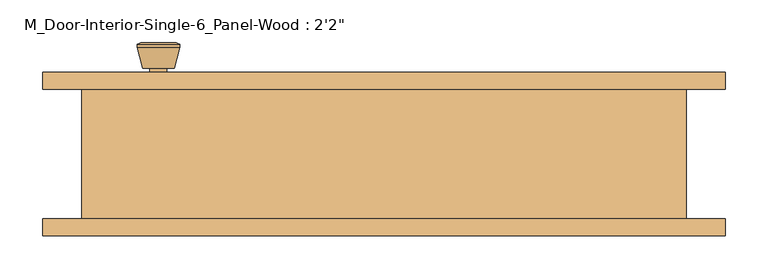
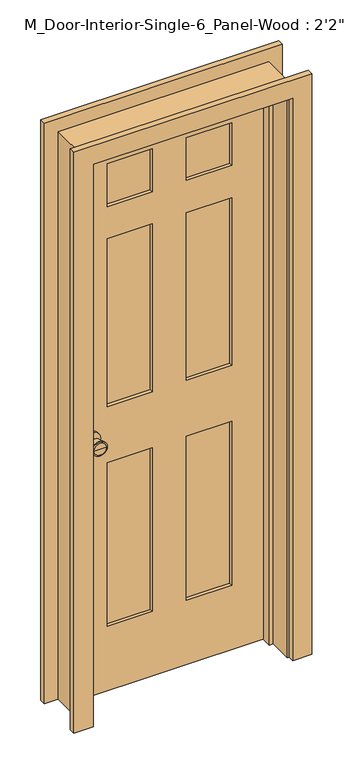
"""IFC4 building model written with IfcOpenShell, lengths in millimetres: door geometry."""

from ifc_helpers import new_model, si_unit, point, frame, frame_2d, origin, place, context, project, spatial, polyline, circle_curve, trimmed, segment, composite_curve, outline, extrude, faceted_brep, source, transform, mapped, element, save
from ifc_brep_helpers import plane_surface, cylinder_surface, revolved_surface, advanced_brep


def door_c4e61f94(model_context):
    return source(origin(), model_context, "Body", "SolidModel", [
        advanced_brep(
        [(-265.2, 32.025, 914.4), (-255.2, 32.025, 914.4), (-275.2, 32.025, 914.4), (-244.7241324, -16.975, 914.4), (-265.2, -16.975, 914.4), (-285.6758676, -16.975, 914.4), (-240.2, -15.1471319, 914.4), (-290.2, -15.1471319, 914.4), (-240.2, -11.6834537, 914.4), (-290.2, -11.6834537, 914.4), (-246.563764, 13.025, 914.4), (-283.836236, 13.025, 914.4), (-255.2, 13.025, 914.4), (-275.2, 13.025, 914.4)],
        [
            (0, 1),
            (1, 2, circle_curve(frame((-265.2, 32.025, 914.4), z_axis=(0.0, 1.0, 0.0), x_axis=(-1.0, 0.0, 0.0)), 10.0)),
            (2, 0),
            (2, 1, circle_curve(frame((-265.2, 32.025, 914.4), z_axis=(0.0, 1.0, 0.0), x_axis=(-1.0, 0.0, 0.0)), 10.0)),
            (3, 4),
            (4, 5),
            (5, 3, circle_curve(frame((-265.2, -16.975, 914.4), z_axis=(0.0, -1.0, 0.0), x_axis=(-1.0, 0.0, 0.0)), 20.4758676)),
            (3, 5, circle_curve(frame((-265.2, -16.975, 914.4), z_axis=(0.0, -1.0, 0.0), x_axis=(-1.0, 0.0, 0.0)), 20.4758676)),
            (6, 3),
            (5, 7),
            (7, 6, circle_curve(frame((-265.2, -15.1471319, 914.4), z_axis=(0.0, -1.0, 0.0), x_axis=(-1.0, 0.0, 0.0)), 25.0)),
            (6, 7, circle_curve(frame((-265.2, -15.1471319, 914.4), z_axis=(0.0, -1.0, 0.0), x_axis=(-1.0, 0.0, 0.0)), 25.0)),
            (8, 6),
            (7, 9),
            (9, 8, circle_curve(frame((-265.2, -11.6834537, 914.4), z_axis=(0.0, -1.0, 0.0), x_axis=(-1.0, 0.0, 0.0)), 25.0)),
            (8, 9, circle_curve(frame((-265.2, -11.6834537, 914.4), z_axis=(0.0, -1.0, 0.0), x_axis=(-1.0, 0.0, 0.0)), 25.0)),
            (10, 8),
            (9, 11),
            (11, 10, circle_curve(frame((-265.2, 13.025, 914.4), z_axis=(0.0, -1.0, 0.0), x_axis=(-1.0, 0.0, 0.0)), 18.636236)),
            (10, 11, circle_curve(frame((-265.2, 13.025, 914.4), z_axis=(0.0, -1.0, 0.0), x_axis=(-1.0, 0.0, 0.0)), 18.636236)),
            (12, 10),
            (11, 13),
            (13, 12, circle_curve(frame((-265.2, 13.025, 914.4), z_axis=(0.0, -1.0, 0.0), x_axis=(-1.0, 0.0, 0.0)), 10.0)),
            (12, 13, circle_curve(frame((-265.2, 13.025, 914.4), z_axis=(0.0, -1.0, 0.0), x_axis=(-1.0, 0.0, 0.0)), 10.0)),
            (1, 12),
            (13, 2),
        ],
        [
            plane_surface(frame((-265.2, 32.025, 914.4), z_axis=(0.0, 1.0, 0.0), x_axis=(-1.0, 0.0, 0.0))),
            plane_surface(frame((-265.2, -16.975, 914.4), z_axis=(0.0, -1.0, 0.0), x_axis=(-1.0, 0.0, 0.0))),
            revolved_surface(polyline([(-285.6758676, -16.975, 914.4), (-290.2, -15.1471319, 914.4)]), (-265.2, 32.025, 914.4), (0.0, 1.0, 0.0)),
            cylinder_surface(frame((-265.2, 32.025, 914.4), z_axis=(0.0, 1.0, 0.0), x_axis=(-1.0, 0.0, 0.0)), 25.0),
            revolved_surface(polyline([(-290.2, -11.6834537, 914.4), (-283.836236, 13.025, 914.4)]), (-265.2, 32.025, 914.4), (0.0, 1.0, 0.0)),
            plane_surface(frame((-265.2, 13.025, 914.4), z_axis=(0.0, 1.0, 0.0), x_axis=(-1.0, 0.0, 0.0))),
            cylinder_surface(frame((-265.2, 32.025, 914.4), z_axis=(0.0, 1.0, 0.0), x_axis=(-1.0, 0.0, 0.0)), 10.0),
        ],
        [
            (0, [[1, 2, 3]]),
            (0, [[-3, 4, -1]]),
            (1, [[5, 6, 7]]),
            (1, [[-6, -5, 8]]),
            (2, [[9, -7, 10, 11]]),
            (2, [[-10, -8, -9, 12]]),
            (3, [[13, -11, 14, 15]]),
            (3, [[-14, -12, -13, 16]]),
            (4, [[17, -15, 18, 19]]),
            (4, [[-18, -16, -17, 20]]),
            (5, [[21, -19, 22, 23]]),
            (5, [[-22, -20, -21, 24]]),
            (6, [[25, -23, 26, -2]]),
            (6, [[-26, -24, -25, -4]]),
        ],
    ),
        extrude(outline(composite_curve([segment(trimmed(circle_curve(frame_2d((914.4, -265.2)), 30.0), [point((914.4, -295.2))], [point((914.4, -235.2))], False, "CARTESIAN"), True, "CONTINUOUS"), segment(trimmed(circle_curve(frame_2d((914.4, -265.2)), 30.0), [point((914.4, -235.2))], [point((914.4, -295.2))], False, "CARTESIAN"), True, "CONTINUOUS")], self_intersect=False)), frame((0.0, 32.025, 0.0), z_axis=(0.0, 1.0, 0.0), x_axis=(0.0, 0.0, 1.0)), (0.0, 0.0, 1.0), 6.0),
        advanced_brep(
        [(-265.2, 79.025, 914.4), (-275.2, 79.025, 914.4), (-255.2, 79.025, 914.4), (-244.7241324, 128.025, 914.4), (-285.6758676, 128.025, 914.4), (-265.2, 128.025, 914.4), (-240.2, 126.1971319, 914.4), (-290.2, 126.1971319, 914.4), (-240.2, 122.7334537, 914.4), (-290.2, 122.7334537, 914.4), (-246.563764, 98.025, 914.4), (-283.836236, 98.025, 914.4), (-255.2, 98.025, 914.4), (-275.2, 98.025, 914.4)],
        [
            (0, 1),
            (1, 2, circle_curve(frame((-265.2, 79.025, 914.4), z_axis=(0.0, -1.0, 0.0), x_axis=(-1.0, 0.0, 0.0)), 10.0)),
            (2, 0),
            (2, 1, circle_curve(frame((-265.2, 79.025, 914.4), z_axis=(0.0, -1.0, 0.0), x_axis=(-1.0, 0.0, 0.0)), 10.0)),
            (3, 4, circle_curve(frame((-265.2, 128.025, 914.4), z_axis=(0.0, 1.0, 0.0), x_axis=(-1.0, 0.0, 0.0)), 20.4758676)),
            (4, 5),
            (5, 3),
            (4, 3, circle_curve(frame((-265.2, 128.025, 914.4), z_axis=(0.0, 1.0, 0.0), x_axis=(-1.0, 0.0, 0.0)), 20.4758676)),
            (6, 7, circle_curve(frame((-265.2, 126.1971319, 914.4), z_axis=(0.0, 1.0, 0.0), x_axis=(-1.0, 0.0, 0.0)), 25.0)),
            (7, 4),
            (3, 6),
            (7, 6, circle_curve(frame((-265.2, 126.1971319, 914.4), z_axis=(0.0, 1.0, 0.0), x_axis=(-1.0, 0.0, 0.0)), 25.0)),
            (8, 9, circle_curve(frame((-265.2, 122.7334537, 914.4), z_axis=(0.0, 1.0, 0.0), x_axis=(-1.0, 0.0, 0.0)), 25.0)),
            (9, 7),
            (6, 8),
            (9, 8, circle_curve(frame((-265.2, 122.7334537, 914.4), z_axis=(0.0, 1.0, 0.0), x_axis=(-1.0, 0.0, 0.0)), 25.0)),
            (10, 11, circle_curve(frame((-265.2, 98.025, 914.4), z_axis=(0.0, 1.0, 0.0), x_axis=(-1.0, 0.0, 0.0)), 18.636236)),
            (11, 9),
            (8, 10),
            (11, 10, circle_curve(frame((-265.2, 98.025, 914.4), z_axis=(0.0, 1.0, 0.0), x_axis=(-1.0, 0.0, 0.0)), 18.636236)),
            (12, 13, circle_curve(frame((-265.2, 98.025, 914.4), z_axis=(0.0, 1.0, 0.0), x_axis=(-1.0, 0.0, 0.0)), 10.0)),
            (13, 11),
            (10, 12),
            (13, 12, circle_curve(frame((-265.2, 98.025, 914.4), z_axis=(0.0, 1.0, 0.0), x_axis=(-1.0, 0.0, 0.0)), 10.0)),
            (1, 13),
            (12, 2),
        ],
        [
            plane_surface(frame((-265.2, 79.025, 914.4), z_axis=(0.0, -1.0, 0.0), x_axis=(-1.0, 0.0, 0.0))),
            plane_surface(frame((-265.2, 128.025, 914.4), z_axis=(0.0, 1.0, 0.0), x_axis=(-1.0, 0.0, 0.0))),
            revolved_surface(polyline([(-285.6758676, 128.025, 914.4), (-290.2, 126.1971319, 914.4)]), (-265.2, 79.025, 914.4), (0.0, -1.0, 0.0)),
            cylinder_surface(frame((-265.2, 79.025, 914.4), z_axis=(0.0, -1.0, 0.0), x_axis=(-1.0, 0.0, 0.0)), 25.0),
            revolved_surface(polyline([(-290.2, 122.7334537, 914.4), (-283.836236, 98.025, 914.4)]), (-265.2, 79.025, 914.4), (0.0, -1.0, 0.0)),
            plane_surface(frame((-265.2, 98.025, 914.4), z_axis=(0.0, -1.0, 0.0), x_axis=(-1.0, 0.0, 0.0))),
            cylinder_surface(frame((-265.2, 79.025, 914.4), z_axis=(0.0, -1.0, 0.0), x_axis=(-1.0, 0.0, 0.0)), 10.0),
        ],
        [
            (0, [[1, 2, 3]]),
            (0, [[-3, 4, -1]]),
            (1, [[5, 6, 7]]),
            (1, [[8, -7, -6]]),
            (2, [[9, 10, -5, 11]]),
            (2, [[12, -11, -8, -10]]),
            (3, [[13, 14, -9, 15]]),
            (3, [[16, -15, -12, -14]]),
            (4, [[17, 18, -13, 19]]),
            (4, [[20, -19, -16, -18]]),
            (5, [[21, 22, -17, 23]]),
            (5, [[24, -23, -20, -22]]),
            (6, [[-2, 25, -21, 26]]),
            (6, [[-4, -26, -24, -25]]),
        ],
    ),
        extrude(outline(composite_curve([segment(trimmed(circle_curve(frame_2d((914.4, -265.2)), 30.0), [point((914.4, -295.2))], [point((914.4, -235.2))], False, "CARTESIAN"), True, "CONTINUOUS"), segment(trimmed(circle_curve(frame_2d((914.4, -265.2)), 30.0), [point((914.4, -235.2))], [point((914.4, -295.2))], False, "CARTESIAN"), True, "CONTINUOUS")], self_intersect=False)), frame((0.0, 73.025, 0.0), z_axis=(0.0, 1.0, 0.0), x_axis=(0.0, 0.0, 1.0)), (0.0, 0.0, 1.0), 6.0),
        faceted_brep([(355.2, 73.025, 0.0), (355.2, -79.375, 0.0), (330.2, -79.375, 0.0), (330.2, 3.1, 0.0), (317.5, 3.1, 0.0), (317.5, 38.025, 0.0), (330.2, 38.025, 0.0), (330.2, 73.025, 0.0), (355.2, 73.025, 2025.0), (355.2, -79.375, 2025.0), (-355.2, -79.375, 2025.0), (-355.2, -79.375, 0.0), (-330.2, -79.375, 0.0), (-330.2, -79.375, 2000.0), (330.2, -79.375, 2000.0), (330.2, 3.1, 2000.0), (-330.2, 3.1, 2000.0), (-330.2, 3.1, 0.0), (-317.5, 3.1, 0.0), (-317.5, 3.1, 1987.3), (317.5, 3.1, 1987.3), (317.5, 38.025, 1987.3), (-317.5, 38.025, 1987.3), (-317.5, 38.025, 0.0), (-330.2, 38.025, 0.0), (-330.2, 38.025, 2000.0), (330.2, 38.025, 2000.0), (330.2, 73.025, 2000.0), (-330.2, 73.025, 2000.0), (-330.2, 73.025, 0.0), (-355.2, 73.025, 0.0), (-355.2, 73.025, 2025.0)], [[[0, 1, 2, 3, 4, 5, 6, 7]], [[1, 0, 8, 9]], [[2, 1, 9, 10, 11, 12, 13, 14]], [[3, 2, 14, 15]], [[4, 3, 15, 16, 17, 18, 19, 20]], [[5, 4, 20, 21]], [[6, 5, 21, 22, 23, 24, 25, 26]], [[7, 6, 26, 27]], [[0, 7, 27, 28, 29, 30, 31, 8]], [[9, 8, 31, 10]], [[15, 14, 13, 16]], [[21, 20, 19, 22]], [[27, 26, 25, 28]], [[30, 29, 24, 23, 18, 17, 12, 11]], [[10, 31, 30, 11]], [[16, 13, 12, 17]], [[22, 19, 18, 23]], [[28, 25, 24, 29]]]),
        extrude(outline(polyline([(2000.0, -330.2), (0.0, -330.2), (0.0, 330.2), (2000.0, 330.2), (2000.0, -330.2)]), holes=[polyline([(1880.0, 57.5), (1880.0, 210.2), (1727.3, 210.2), (1727.3, 57.5), (1880.0, 57.5)]), polyline([(1612.3, 210.2), (1014.4, 210.2), (1014.4, 57.5), (1612.3, 57.5), (1612.3, 210.2)]), polyline([(1014.4, -57.5), (1014.4, -210.2), (1612.3, -210.2), (1612.3, -57.5), (1014.4, -57.5)]), polyline([(1727.3, -210.2), (1880.0, -210.2), (1880.0, -57.5), (1727.3, -57.5), (1727.3, -210.2)]), polyline([(814.4, 57.5), (814.4, 210.2), (230.0, 210.2), (230.0, 57.5), (814.4, 57.5)]), polyline([(230.0, -57.5), (230.0, -210.2), (814.4, -210.2), (814.4, -57.5), (230.0, -57.5)])]), frame((0.0, 38.025, 0.0), z_axis=(0.0, 1.0, 0.0), x_axis=(0.0, 0.0, 1.0)), (0.0, 0.0, 1.0), 35.0),
        extrude(outline(polyline([(210.2, 49.6916667), (57.5, 49.6916667), (57.5, 61.3583333), (210.2, 61.3583333), (210.2, 49.6916667)])), frame((0.0, 0.0, 1727.3), z_axis=(0.0, 0.0, 1.0), x_axis=(1.0, 0.0, 0.0)), (0.0, 0.0, 1.0), 152.7),
        extrude(outline(polyline([(210.2, 49.6916667), (57.5, 49.6916667), (57.5, 61.3583333), (210.2, 61.3583333), (210.2, 49.6916667)])), frame((0.0, 0.0, 1014.4), z_axis=(0.0, 0.0, 1.0), x_axis=(1.0, 0.0, 0.0)), (0.0, 0.0, 1.0), 597.9),
        extrude(outline(polyline([(-57.5, 49.6916667), (-210.2, 49.6916667), (-210.2, 61.3583333), (-57.5, 61.3583333), (-57.5, 49.6916667)])), frame((0.0, 0.0, 1014.4), z_axis=(0.0, 0.0, 1.0), x_axis=(1.0, 0.0, 0.0)), (0.0, 0.0, 1.0), 597.9),
        extrude(outline(polyline([(-57.5, 49.6916667), (-210.2, 49.6916667), (-210.2, 61.3583333), (-57.5, 61.3583333), (-57.5, 49.6916667)])), frame((0.0, 0.0, 1727.3), z_axis=(0.0, 0.0, 1.0), x_axis=(1.0, 0.0, 0.0)), (0.0, 0.0, 1.0), 152.7),
        extrude(outline(polyline([(210.2, 49.6916667), (57.5, 49.6916667), (57.5, 61.3583333), (210.2, 61.3583333), (210.2, 49.6916667)])), frame((0.0, 0.0, 230.0), z_axis=(0.0, 0.0, 1.0), x_axis=(1.0, 0.0, 0.0)), (0.0, 0.0, 1.0), 584.4),
        extrude(outline(polyline([(-57.5, 49.6916667), (-210.2, 49.6916667), (-210.2, 61.3583333), (-57.5, 61.3583333), (-57.5, 49.6916667)])), frame((0.0, 0.0, 230.0), z_axis=(0.0, 0.0, 1.0), x_axis=(1.0, 0.0, 0.0)), (0.0, 0.0, 1.0), 584.4),
        extrude(outline(polyline([(0.0, 336.55), (0.0, 401.55), (2071.35, 401.55), (2071.35, -401.55), (0.0, -401.55), (0.0, -336.55), (2006.35, -336.55), (2006.35, 336.55), (0.0, 336.55)])), frame((0.0, 73.025, 0.0), z_axis=(0.0, 1.0, 0.0), x_axis=(0.0, 0.0, 1.0)), (0.0, 0.0, 1.0), 20.0),
        extrude(outline(polyline([(0.0, 336.55), (0.0, 401.55), (2071.35, 401.55), (2071.35, -401.55), (0.0, -401.55), (0.0, -336.55), (2006.35, -336.55), (2006.35, 336.55), (0.0, 336.55)])), frame((0.0, -99.375, 0.0), z_axis=(0.0, 1.0, 0.0), x_axis=(0.0, 0.0, 1.0)), (0.0, 0.0, 1.0), 20.0),
    ])


if __name__ == "__main__":
    model = new_model("IFC4")
    model_context = context("Model", 3, world=origin())
    ifc_project = project(units=[si_unit("LENGTHUNIT", "METRE", prefix="MILLI")], contexts=[model_context])
    site = spatial("IfcSite", under=ifc_project)
    building = spatial("IfcBuilding", under=site)
    placement = place(None, origin())
    door_shape = door_c4e61f94(model_context)
    element("IfcDoor", 1, ObjectType="M_Door-Interior-Single-6_Panel-Wood : 2'2\"", at=placement, inside=building, context=model_context, shape_type="MappedRepresentation", body=[
        mapped(door_shape, transform((0.0, 0.0, 0.0), x_axis=(1.0, 0.0, 0.0), y_axis=(0.0, 1.0, 0.0), z_axis=(0.0, 0.0, 1.0))),
    ])
    save(model, "model.ifc")

# Revit data of these elements
# Type "M_Door-Interior-Single-6_Panel-Wood : 2'2\""
#   Type Mark = "47"
#   Assembly Code = "C1020300"
#   Analytic Construction = "Wooden"
#   Top Rail = 0' - 4.72441"
#   Top Panel = 0' - 6.01181"
#   Thickness = 0' - 1.37795"
#   Thermal Resistance (R) = 0.455703 (m²·K)/W
#   Swing Angle [instance default] = 90.00°
#   Stiles = 0' - 4.72441"
#   Rough Width = 2' - 3.9685"
#   Rough Height = 6' - 7.72441"
#   Mullion = 0' - 4.52756"
#   Lock Rail = 0' - 7.87402"
#   Intermediate Rail = 0' - 4.52756"
#   Height = 6' - 6.74016"
#   Width = 2' - 2"
#   Heat Transfer Coefficient (U) = 2.19465 W/(m²·K)
#   Bottom Rail = 0' - 9.05512"
#   Trim Material = Cherry
#   Panel Material = Cherry
#   Frame Material = Cherry
#   Door Handle Material = Aluminum
#   Visual Light Transmittance = 0
#   Solar Heat Gain Coefficient = 0
#   Wall Closure = (empty or 0)
#   Function = (empty or 0)
# Element 1 (IfcDoor, "M_Door-Interior-Single-6_Panel-Wood : 2'2\"")
#   Materials on its faces: "Cherry", "Aluminum"
# Materials
#   "Cherry": class "Wood", colour RGB 226 177 128, transparency 0, Description = "Prunus Serotina", Cost = 0
#   "Aluminum": class "Metal", colour RGB 247 247 247, transparency 0, Description = "Aluminum 6061", Cost = 0
